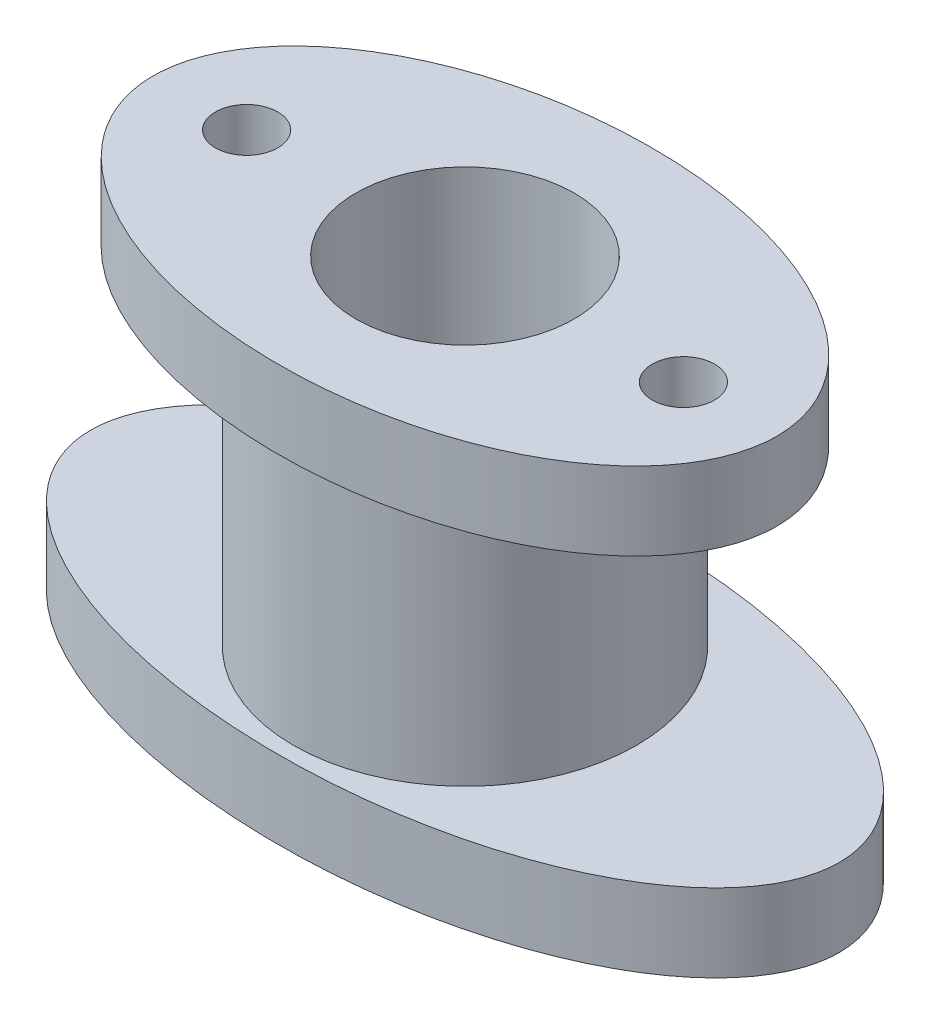
ISO-10303-21;
HEADER;
FILE_DESCRIPTION(('STEP AP214'),'2;1');
FILE_NAME('part.step','',(''),(''),'','','');
FILE_SCHEMA(('AUTOMOTIVE_DESIGN { 1 0 10303 214 1 1 1 1 }'));
ENDSEC;
DATA;
#1=APPLICATION_CONTEXT('core data for automotive mechanical design processes');
#2=APPLICATION_PROTOCOL_DEFINITION('international standard','automotive_design',2000,#1);
#3=PRODUCT_CONTEXT('',#1,'mechanical');
#4=PRODUCT('Part','Part','',(#3));
#5=PRODUCT_RELATED_PRODUCT_CATEGORY('part','',(#4));
#6=PRODUCT_DEFINITION_FORMATION('','',#4);
#7=PRODUCT_DEFINITION_CONTEXT('part definition',#1,'design');
#8=PRODUCT_DEFINITION('design','',#6,#7);
#9=PRODUCT_DEFINITION_SHAPE('','',#8);
#10=(LENGTH_UNIT() NAMED_UNIT(*) SI_UNIT(.MILLI.,.METRE.));
#11=(NAMED_UNIT(*) PLANE_ANGLE_UNIT() SI_UNIT($,.RADIAN.));
#12=(NAMED_UNIT(*) SI_UNIT($,.STERADIAN.) SOLID_ANGLE_UNIT());
#13=UNCERTAINTY_MEASURE_WITH_UNIT(LENGTH_MEASURE(1.E-05),#10,'distance_accuracy_value','');
#14=(GEOMETRIC_REPRESENTATION_CONTEXT(3) GLOBAL_UNCERTAINTY_ASSIGNED_CONTEXT((#13)) GLOBAL_UNIT_ASSIGNED_CONTEXT((#10,
#11,#12)) REPRESENTATION_CONTEXT('',''));
#15=CARTESIAN_POINT('',(0.,0.,0.));
#16=DIRECTION('',(0.,0.,1.));
#17=DIRECTION('',(1.,0.,0.));
#18=AXIS2_PLACEMENT_3D('',#15,#16,#17);
#19=CARTESIAN_POINT('',(0.,15.,0.));
#20=DIRECTION('',(0.,1.,0.));
#21=DIRECTION('',(1.,0.,0.));
#22=AXIS2_PLACEMENT_3D('',#19,#20,#21);
#23=ELLIPSE('',#22,72.,36.);
#24=DIRECTION('',(0.,-1.,0.));
#25=VECTOR('',#24,1.);
#26=SURFACE_OF_LINEAR_EXTRUSION('',#23,#25);
#27=CARTESIAN_POINT('',(72.,15.,0.));
#28=VERTEX_POINT('',#27);
#29=EDGE_CURVE('E10',#28,#28,#23,.T.);
#30=ORIENTED_EDGE('',*,*,#29,.F.);
#31=EDGE_LOOP('',(#30));
#32=FACE_BOUND('',#31,.T.);
#33=CARTESIAN_POINT('',(0.,0.,0.));
#34=DIRECTION('',(0.,1.,0.));
#35=DIRECTION('',(1.,0.,0.));
#36=AXIS2_PLACEMENT_3D('',#33,#34,#35);
#37=ELLIPSE('',#36,72.,36.);
#38=CARTESIAN_POINT('',(72.,0.,0.));
#39=VERTEX_POINT('',#38);
#40=EDGE_CURVE('E41',#39,#39,#37,.T.);
#41=ORIENTED_EDGE('',*,*,#40,.T.);
#42=EDGE_LOOP('',(#41));
#43=FACE_BOUND('',#42,.T.);
#44=ADVANCED_FACE('F40',(#32,#43),#26,.F.);
#45=CARTESIAN_POINT('',(0.,15.,0.));
#46=DIRECTION('',(0.,1.,0.));
#47=DIRECTION('',(0.,0.,1.));
#48=AXIS2_PLACEMENT_3D('',#45,#46,#47);
#49=PLANE('',#48);
#50=CARTESIAN_POINT('',(0.,15.,0.));
#51=DIRECTION('',(0.,1.,0.));
#52=DIRECTION('',(0.,0.,1.));
#53=AXIS2_PLACEMENT_3D('',#50,#51,#52);
#54=CIRCLE('',#53,33.);
#55=CARTESIAN_POINT('',(0.,15.,33.));
#56=VERTEX_POINT('',#55);
#57=EDGE_CURVE('E49',#56,#56,#54,.T.);
#58=ORIENTED_EDGE('',*,*,#57,.F.);
#59=EDGE_LOOP('',(#58));
#60=FACE_BOUND('',#59,.T.);
#61=ORIENTED_EDGE('',*,*,#29,.T.);
#62=EDGE_LOOP('',(#61));
#63=FACE_BOUND('',#62,.T.);
#64=ADVANCED_FACE('F78',(#60,#63),#49,.T.);
#65=CARTESIAN_POINT('',(0.,0.,0.));
#66=DIRECTION('',(0.,1.,0.));
#67=DIRECTION('',(0.,0.,1.));
#68=AXIS2_PLACEMENT_3D('',#65,#66,#67);
#69=PLANE('',#68);
#70=ORIENTED_EDGE('',*,*,#40,.F.);
#71=EDGE_LOOP('',(#70));
#72=FACE_BOUND('',#71,.T.);
#73=ADVANCED_FACE('F80',(#72),#69,.F.);
#74=CARTESIAN_POINT('',(0.,65.,0.));
#75=DIRECTION('',(0.,-1.,0.));
#76=DIRECTION('',(0.,0.,-1.));
#77=AXIS2_PLACEMENT_3D('',#74,#75,#76);
#78=CYLINDRICAL_SURFACE('',#77,33.);
#79=CARTESIAN_POINT('',(0.,65.,0.));
#80=DIRECTION('',(0.,1.,0.));
#81=DIRECTION('',(0.,0.,1.));
#82=AXIS2_PLACEMENT_3D('',#79,#80,#81);
#83=CIRCLE('',#82,33.);
#84=CARTESIAN_POINT('',(0.,65.,33.));
#85=VERTEX_POINT('',#84);
#86=EDGE_CURVE('E50',#85,#85,#83,.T.);
#87=ORIENTED_EDGE('',*,*,#86,.F.);
#88=EDGE_LOOP('',(#87));
#89=FACE_BOUND('',#88,.T.);
#90=ORIENTED_EDGE('',*,*,#57,.T.);
#91=EDGE_LOOP('',(#90));
#92=FACE_BOUND('',#91,.T.);
#93=ADVANCED_FACE('F74',(#89,#92),#78,.T.);
#94=CARTESIAN_POINT('',(0.,80.,0.));
#95=DIRECTION('',(0.,1.,0.));
#96=DIRECTION('',(0.,0.,1.));
#97=AXIS2_PLACEMENT_3D('',#94,#95,#96);
#98=PLANE('',#97);
#99=CARTESIAN_POINT('',(0.,80.,0.));
#100=DIRECTION('',(0.,1.,0.));
#101=DIRECTION('',(0.,0.,1.));
#102=AXIS2_PLACEMENT_3D('',#99,#100,#101);
#103=CIRCLE('',#102,21.);
#104=CARTESIAN_POINT('',(0.,80.,21.));
#105=VERTEX_POINT('',#104);
#106=EDGE_CURVE('E178',#105,#105,#103,.T.);
#107=ORIENTED_EDGE('',*,*,#106,.F.);
#108=EDGE_LOOP('',(#107));
#109=FACE_BOUND('',#108,.T.);
#110=CARTESIAN_POINT('',(-42.,80.,0.));
#111=DIRECTION('',(0.,1.,0.));
#112=DIRECTION('',(0.,0.,1.));
#113=AXIS2_PLACEMENT_3D('',#110,#111,#112);
#114=CIRCLE('',#113,5.99999999999999);
#115=CARTESIAN_POINT('',(-42.,80.,5.99999999999999));
#116=VERTEX_POINT('',#115);
#117=EDGE_CURVE('E56',#116,#116,#114,.T.);
#118=ORIENTED_EDGE('',*,*,#117,.F.);
#119=EDGE_LOOP('',(#118));
#120=FACE_BOUND('',#119,.T.);
#121=CARTESIAN_POINT('',(0.,80.,0.));
#122=DIRECTION('',(0.,1.,0.));
#123=DIRECTION('',(1.,0.,0.));
#124=AXIS2_PLACEMENT_3D('',#121,#122,#123);
#125=ELLIPSE('',#124,60.,36.);
#126=CARTESIAN_POINT('',(60.,80.,0.));
#127=VERTEX_POINT('',#126);
#128=EDGE_CURVE('E52',#127,#127,#125,.T.);
#129=ORIENTED_EDGE('',*,*,#128,.T.);
#130=EDGE_LOOP('',(#129));
#131=FACE_BOUND('',#130,.T.);
#132=CARTESIAN_POINT('',(42.,80.,0.));
#133=DIRECTION('',(0.,1.,0.));
#134=DIRECTION('',(0.,0.,1.));
#135=AXIS2_PLACEMENT_3D('',#132,#133,#134);
#136=CIRCLE('',#135,5.99999999999999);
#137=CARTESIAN_POINT('',(42.,80.,5.99999999999999));
#138=VERTEX_POINT('',#137);
#139=EDGE_CURVE('E182',#138,#138,#136,.T.);
#140=ORIENTED_EDGE('',*,*,#139,.F.);
#141=EDGE_LOOP('',(#140));
#142=FACE_BOUND('',#141,.T.);
#143=ADVANCED_FACE('F79',(#109,#120,#131,#142),#98,.T.);
#144=CARTESIAN_POINT('',(0.,65.,0.));
#145=DIRECTION('',(0.,1.,0.));
#146=DIRECTION('',(0.,0.,1.));
#147=AXIS2_PLACEMENT_3D('',#144,#145,#146);
#148=PLANE('',#147);
#149=ORIENTED_EDGE('',*,*,#86,.T.);
#150=EDGE_LOOP('',(#149));
#151=FACE_BOUND('',#150,.T.);
#152=CARTESIAN_POINT('',(0.,65.,0.));
#153=DIRECTION('',(0.,1.,0.));
#154=DIRECTION('',(1.,0.,0.));
#155=AXIS2_PLACEMENT_3D('',#152,#153,#154);
#156=ELLIPSE('',#155,60.,36.);
#157=CARTESIAN_POINT('',(60.,65.,0.));
#158=VERTEX_POINT('',#157);
#159=EDGE_CURVE('E57',#158,#158,#156,.T.);
#160=ORIENTED_EDGE('',*,*,#159,.F.);
#161=EDGE_LOOP('',(#160));
#162=FACE_BOUND('',#161,.T.);
#163=CARTESIAN_POINT('',(-42.,65.,0.));
#164=DIRECTION('',(0.,1.,0.));
#165=DIRECTION('',(0.,0.,1.));
#166=AXIS2_PLACEMENT_3D('',#163,#164,#165);
#167=CIRCLE('',#166,5.99999999999999);
#168=CARTESIAN_POINT('',(-42.,65.,5.99999999999999));
#169=VERTEX_POINT('',#168);
#170=EDGE_CURVE('E65',#169,#169,#167,.T.);
#171=ORIENTED_EDGE('',*,*,#170,.T.);
#172=EDGE_LOOP('',(#171));
#173=FACE_BOUND('',#172,.T.);
#174=CARTESIAN_POINT('',(42.,65.,0.));
#175=DIRECTION('',(0.,1.,0.));
#176=DIRECTION('',(0.,0.,1.));
#177=AXIS2_PLACEMENT_3D('',#174,#175,#176);
#178=CIRCLE('',#177,5.99999999999999);
#179=CARTESIAN_POINT('',(42.,65.,5.99999999999999));
#180=VERTEX_POINT('',#179);
#181=EDGE_CURVE('E180',#180,#180,#178,.T.);
#182=ORIENTED_EDGE('',*,*,#181,.T.);
#183=EDGE_LOOP('',(#182));
#184=FACE_BOUND('',#183,.T.);
#185=ADVANCED_FACE('F72',(#151,#162,#173,#184),#148,.F.);
#186=DIRECTION('',(0.,-1.,0.));
#187=VECTOR('',#186,1.);
#188=SURFACE_OF_LINEAR_EXTRUSION('',#125,#187);
#189=ORIENTED_EDGE('',*,*,#128,.F.);
#190=EDGE_LOOP('',(#189));
#191=FACE_BOUND('',#190,.T.);
#192=ORIENTED_EDGE('',*,*,#159,.T.);
#193=EDGE_LOOP('',(#192));
#194=FACE_BOUND('',#193,.T.);
#195=ADVANCED_FACE('F66',(#191,#194),#188,.F.);
#196=CARTESIAN_POINT('',(-42.,80.,0.));
#197=DIRECTION('',(0.,-1.,0.));
#198=DIRECTION('',(0.,0.,-1.));
#199=AXIS2_PLACEMENT_3D('',#196,#197,#198);
#200=CYLINDRICAL_SURFACE('',#199,5.99999999999999);
#201=ORIENTED_EDGE('',*,*,#117,.T.);
#202=EDGE_LOOP('',(#201));
#203=FACE_BOUND('',#202,.T.);
#204=ORIENTED_EDGE('',*,*,#170,.F.);
#205=EDGE_LOOP('',(#204));
#206=FACE_BOUND('',#205,.T.);
#207=ADVANCED_FACE('F69',(#203,#206),#200,.F.);
#208=CARTESIAN_POINT('',(42.,80.,0.));
#209=DIRECTION('',(0.,-1.,0.));
#210=DIRECTION('',(0.,0.,-1.));
#211=AXIS2_PLACEMENT_3D('',#208,#209,#210);
#212=CYLINDRICAL_SURFACE('',#211,5.99999999999999);
#213=ORIENTED_EDGE('',*,*,#139,.T.);
#214=EDGE_LOOP('',(#213));
#215=FACE_BOUND('',#214,.T.);
#216=ORIENTED_EDGE('',*,*,#181,.F.);
#217=EDGE_LOOP('',(#216));
#218=FACE_BOUND('',#217,.T.);
#219=ADVANCED_FACE('F141',(#215,#218),#212,.F.);
#220=CARTESIAN_POINT('',(0.,15.,0.));
#221=DIRECTION('',(0.,1.,0.));
#222=DIRECTION('',(0.,0.,1.));
#223=AXIS2_PLACEMENT_3D('',#220,#221,#222);
#224=CYLINDRICAL_SURFACE('',#223,21.);
#225=CARTESIAN_POINT('',(0.,15.,0.));
#226=DIRECTION('',(0.,1.,0.));
#227=DIRECTION('',(0.,0.,1.));
#228=AXIS2_PLACEMENT_3D('',#225,#226,#227);
#229=CIRCLE('',#228,21.);
#230=CARTESIAN_POINT('',(0.,15.,21.));
#231=VERTEX_POINT('',#230);
#232=EDGE_CURVE('E176',#231,#231,#229,.T.);
#233=ORIENTED_EDGE('',*,*,#232,.F.);
#234=EDGE_LOOP('',(#233));
#235=FACE_BOUND('',#234,.T.);
#236=ORIENTED_EDGE('',*,*,#106,.T.);
#237=EDGE_LOOP('',(#236));
#238=FACE_BOUND('',#237,.T.);
#239=ADVANCED_FACE('F155',(#235,#238),#224,.F.);
#240=CARTESIAN_POINT('',(0.,15.,0.));
#241=DIRECTION('',(0.,1.,0.));
#242=DIRECTION('',(0.,0.,1.));
#243=AXIS2_PLACEMENT_3D('',#240,#241,#242);
#244=PLANE('',#243);
#245=ORIENTED_EDGE('',*,*,#232,.T.);
#246=EDGE_LOOP('',(#245));
#247=FACE_BOUND('',#246,.T.);
#248=ADVANCED_FACE('F161',(#247),#244,.T.);
#249=CLOSED_SHELL('',(#44,#64,#73,#93,#143,#185,#195,#207,#219,#239,#248));
#250=MANIFOLD_SOLID_BREP('B2',#249);
#251=ADVANCED_BREP_SHAPE_REPRESENTATION('',(#18,#250),#14);
#252=SHAPE_DEFINITION_REPRESENTATION(#9,#251);
ENDSEC;
END-ISO-10303-21;
